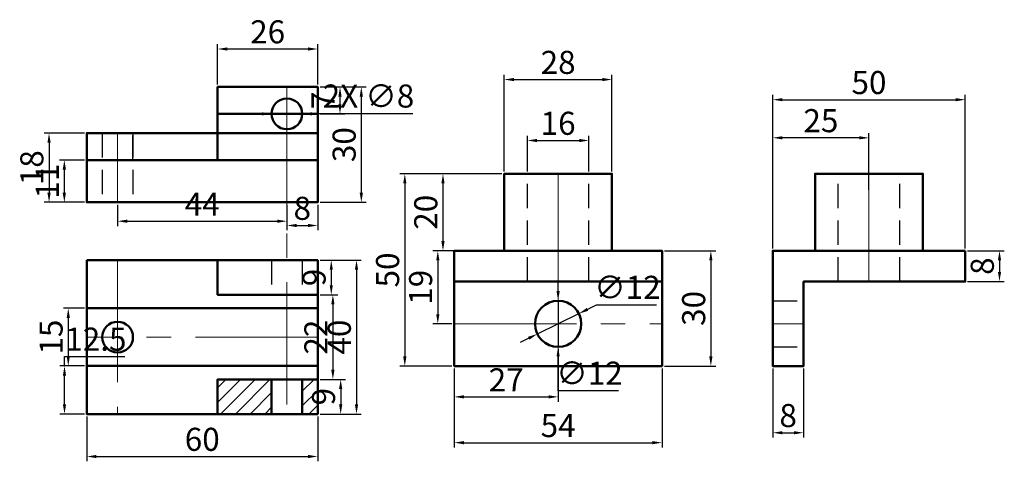
# Model space of a CAD drawing. Units: millimetres. Extents: x 12 to 268, y 574 to 689.
import ezdxf

# ---------------------------------------------------------------- set-up
doc = ezdxf.new("R2010")
doc.units = ezdxf.units.MM
doc.linetypes.add('CENTER', pattern=[50.8, 31.75, -6.35, 6.35, -6.35])
doc.linetypes.add('HIDDEN', pattern=[9.525, 6.35, -3.175])
for name, color, linetype, lineweight in [('M-CNTR', 4, 'CENTER', 18), ('M-DIMS', 2, 'Continuous', 25), ('M-HATC', 8, 'Continuous', 18), ('M-HIDN', 1, 'HIDDEN', 25), ('M-OUTL', 7, 'Continuous', 50)]:
    doc.layers.add(name, color=color, linetype=linetype, lineweight=lineweight)
doc.styles.get("Standard").update_dxf_attribs({"font": 'arial.ttf'})
doc.dimstyles.new('ISO-25', dxfattribs={"dimtxt": 6, "dimasz": 2.5, "dimexe": 1.25, "dimexo": 0.625, "dimtad": 1, "dimtoh": 1, "dimdec": 0, "dimtxsty": 'Standard', "dimcen": 2.5, "dimadec": 0, "dimazin": 0, "dimtfac": 1, "dimtdec": 0, "dimtmove": 0, "dimatfit": 3, "dimfxl": 1, "dimarcsym": 0})

# ---------------------------------------------------------------- blocks, each defined once
blk = doc.blocks.new('*D1')
at = {"layer": 'Defpoints', "color": 0, "transparency": 16777216}
for p in [(89.08, 681.66), (63.08, 671.79), (89.08, 671.79)]:
    blk.add_point(p, dxfattribs=at)
at = {"layer": 'M-DIMS', "color": 0, "lineweight": -2, "transparency": 16777216}
for p, q in [((63.08, 672.42), (63.08, 682.91)), ((65.58, 681.66), (86.58, 681.66)), ((89.08, 672.42), (89.08, 682.91))]:
    blk.add_line(p, q, dxfattribs=at)
at = {"layer": 'M-DIMS', "color": 0, "transparency": 16777216}
for points in [[(65.58, 682.07), (65.58, 681.24), (63.08, 681.66)], [(86.58, 682.07), (86.58, 681.24), (89.08, 681.66)]]:
    blk.add_solid(points, dxfattribs=at)
at = {"layer": 'M-DIMS', "color": 0, "transparency": 16777216, "insert": (76.08, 685.35), "char_height": 6, "attachment_point": 5}
blk.add_mtext('26', dxfattribs=at)
blk = doc.blocks.new('*D2')
at = {"layer": 'Defpoints', "color": 0, "transparency": 16777216}
for p in [(89.08, 671.79), (89.08, 641.79), (100.42, 641.79)]:
    blk.add_point(p, dxfattribs=at)
at = {"layer": 'M-DIMS', "color": 0, "lineweight": -2, "transparency": 16777216}
for p, q in [((89.7, 671.79), (101.67, 671.79)), ((100.42, 669.29), (100.42, 644.29)), ((89.7, 641.79), (101.67, 641.79))]:
    blk.add_line(p, q, dxfattribs=at)
at = {"layer": 'M-DIMS', "color": 0, "transparency": 16777216}
for points in [[(100, 669.29), (100.84, 669.29), (100.42, 671.79)], [(100, 644.29), (100.84, 644.29), (100.42, 641.79)]]:
    blk.add_solid(points, dxfattribs=at)
at = {"layer": 'M-DIMS', "color": 0, "transparency": 16777216, "insert": (96.73, 656.79), "char_height": 6, "attachment_point": 5, "rotation": 90}
blk.add_mtext('30', dxfattribs=at)
blk = doc.blocks.new('*D3')
at = {"layer": 'Defpoints', "color": 0, "transparency": 16777216}
for p in [(29.08, 659.79), (19.26, 641.79), (29.08, 641.79)]:
    blk.add_point(p, dxfattribs=at)
at = {"layer": 'M-DIMS', "color": 0, "lineweight": -2, "transparency": 16777216}
for p, q in [((28.45, 659.79), (18.01, 659.79)), ((19.26, 657.29), (19.26, 644.29)), ((28.45, 641.79), (18.01, 641.79))]:
    blk.add_line(p, q, dxfattribs=at)
at = {"layer": 'M-DIMS', "color": 0, "transparency": 16777216}
for points in [[(18.84, 657.29), (19.68, 657.29), (19.26, 659.79)], [(18.84, 644.29), (19.68, 644.29), (19.26, 641.79)]]:
    blk.add_solid(points, dxfattribs=at)
at = {"layer": 'M-DIMS', "color": 0, "transparency": 16777216, "insert": (15.57, 650.79), "char_height": 6, "attachment_point": 5, "rotation": 90}
blk.add_mtext('18', dxfattribs=at)
blk = doc.blocks.new('*D4')
at = {"layer": 'Defpoints', "color": 0, "transparency": 16777216}
for p in [(29.08, 652.79), (23.23, 641.79), (29.08, 641.79)]:
    blk.add_point(p, dxfattribs=at)
at = {"layer": 'M-DIMS', "color": 0, "lineweight": -2, "transparency": 16777216}
for p, q in [((28.45, 652.79), (21.98, 652.79)), ((23.23, 650.29), (23.23, 644.29)), ((28.45, 641.79), (21.98, 641.79))]:
    blk.add_line(p, q, dxfattribs=at)
at = {"layer": 'M-DIMS', "color": 0, "transparency": 16777216}
for points in [[(22.81, 650.29), (23.65, 650.29), (23.23, 652.79)], [(22.81, 644.29), (23.65, 644.29), (23.23, 641.79)]]:
    blk.add_solid(points, dxfattribs=at)
at = {"layer": 'M-DIMS', "color": 0, "transparency": 16777216, "insert": (19.59, 647.29), "char_height": 6, "attachment_point": 5, "rotation": 90}
blk.add_mtext('11', dxfattribs=at)
blk = doc.blocks.new('*D5')
at = {"layer": 'Defpoints', "color": 0, "transparency": 16777216}
for p in [(37.08, 641.79), (81.08, 641.79), (81.08, 636.88)]:
    blk.add_point(p, dxfattribs=at)
at = {"layer": 'M-DIMS', "color": 0, "lineweight": -2, "transparency": 16777216}
for p, q in [((37.08, 641.17), (37.08, 635.63)), ((81.08, 641.17), (81.08, 635.63)), ((39.58, 636.88), (78.58, 636.88))]:
    blk.add_line(p, q, dxfattribs=at)
at = {"layer": 'M-DIMS', "color": 0, "transparency": 16777216}
for points in [[(39.58, 637.29), (39.58, 636.46), (37.08, 636.88)], [(78.58, 637.29), (78.58, 636.46), (81.08, 636.88)]]:
    blk.add_solid(points, dxfattribs=at)
at = {"layer": 'M-DIMS', "color": 0, "transparency": 16777216, "insert": (59.08, 640.5), "char_height": 6, "attachment_point": 5}
blk.add_mtext('44', dxfattribs=at)
blk = doc.blocks.new('*D6')
at = {"layer": 'Defpoints', "color": 0, "transparency": 16777216}
for p in [(81.08, 641.79), (89.08, 641.79), (89.08, 635.76)]:
    blk.add_point(p, dxfattribs=at)
at = {"layer": 'M-DIMS', "color": 0, "lineweight": -2, "transparency": 16777216}
for p, q in [((81.08, 641.17), (81.08, 634.51)), ((89.08, 641.17), (89.08, 634.51)), ((83.58, 635.76), (86.58, 635.76))]:
    blk.add_line(p, q, dxfattribs=at)
at = {"layer": 'M-DIMS', "color": 0, "transparency": 16777216}
for points in [[(83.58, 636.18), (83.58, 635.35), (81.08, 635.76)], [(86.58, 636.18), (86.58, 635.35), (89.08, 635.76)]]:
    blk.add_solid(points, dxfattribs=at)
at = {"layer": 'M-DIMS', "color": 0, "transparency": 16777216, "insert": (85.08, 639.45), "char_height": 6, "attachment_point": 5}
blk.add_mtext('8', dxfattribs=at)
blk = doc.blocks.new('*D7')
at = {"layer": 'Defpoints', "color": 0, "transparency": 16777216}
for p in [(89.08, 626.74), (89.08, 617.74), (92.61, 617.74)]:
    blk.add_point(p, dxfattribs=at)
at = {"layer": 'M-DIMS', "color": 0, "lineweight": -2, "transparency": 16777216}
for p, q in [((89.7, 626.74), (93.86, 626.74)), ((92.61, 624.24), (92.61, 620.24)), ((89.7, 617.74), (93.86, 617.74))]:
    blk.add_line(p, q, dxfattribs=at)
at = {"layer": 'M-DIMS', "color": 0, "transparency": 16777216}
for points in [[(92.2, 624.24), (93.03, 624.24), (92.61, 626.74)], [(92.2, 620.24), (93.03, 620.24), (92.61, 617.74)]]:
    blk.add_solid(points, dxfattribs=at)
at = {"layer": 'M-DIMS', "color": 0, "transparency": 16777216, "insert": (88.92, 622.24), "char_height": 6, "attachment_point": 5, "rotation": 90}
blk.add_mtext('9', dxfattribs=at)
blk = doc.blocks.new('*D8')
at = {"layer": 'Defpoints', "color": 0, "transparency": 16777216}
for p in [(89.08, 626.74), (89.08, 586.74), (99.17, 586.74)]:
    blk.add_point(p, dxfattribs=at)
at = {"layer": 'M-DIMS', "color": 0, "lineweight": -2, "transparency": 16777216}
for p, q in [((89.7, 626.74), (100.42, 626.74)), ((99.17, 624.24), (99.17, 589.24)), ((89.7, 586.74), (100.42, 586.74))]:
    blk.add_line(p, q, dxfattribs=at)
at = {"layer": 'M-DIMS', "color": 0, "transparency": 16777216}
for points in [[(98.75, 624.24), (99.59, 624.24), (99.17, 626.74)], [(98.75, 589.24), (99.59, 589.24), (99.17, 586.74)]]:
    blk.add_solid(points, dxfattribs=at)
at = {"layer": 'M-DIMS', "color": 0, "transparency": 16777216, "insert": (95.48, 606.74), "char_height": 6, "attachment_point": 5, "rotation": 90}
blk.add_mtext('40', dxfattribs=at)
blk = doc.blocks.new('*D9')
at = {"layer": 'Defpoints', "color": 0, "transparency": 16777216}
for p in [(89.08, 617.74), (89.08, 595.74), (93.03, 595.74)]:
    blk.add_point(p, dxfattribs=at)
at = {"layer": 'M-DIMS', "color": 0, "lineweight": -2, "transparency": 16777216}
for p, q in [((89.7, 617.74), (94.28, 617.74)), ((93.03, 615.24), (93.03, 598.24)), ((89.7, 595.74), (94.28, 595.74))]:
    blk.add_line(p, q, dxfattribs=at)
at = {"layer": 'M-DIMS', "color": 0, "transparency": 16777216}
for points in [[(92.61, 615.24), (93.45, 615.24), (93.03, 617.74)], [(92.61, 598.24), (93.45, 598.24), (93.03, 595.74)]]:
    blk.add_solid(points, dxfattribs=at)
at = {"layer": 'M-DIMS', "color": 0, "transparency": 16777216, "insert": (89.39, 606.74), "char_height": 6, "attachment_point": 5, "rotation": 90}
blk.add_mtext('22', dxfattribs=at)
blk = doc.blocks.new('*D10')
at = {"layer": 'Defpoints', "color": 0, "transparency": 16777216}
for p in [(89.08, 595.74), (89.08, 586.74), (95.06, 586.74)]:
    blk.add_point(p, dxfattribs=at)
at = {"layer": 'M-DIMS', "color": 0, "lineweight": -2, "transparency": 16777216}
for p, q in [((89.7, 595.74), (96.31, 595.74)), ((95.06, 593.24), (95.06, 589.24)), ((89.7, 586.74), (96.31, 586.74))]:
    blk.add_line(p, q, dxfattribs=at)
at = {"layer": 'M-DIMS', "color": 0, "transparency": 16777216}
for points in [[(94.64, 593.24), (95.48, 593.24), (95.06, 595.74)], [(94.64, 589.24), (95.48, 589.24), (95.06, 586.74)]]:
    blk.add_solid(points, dxfattribs=at)
at = {"layer": 'M-DIMS', "color": 0, "transparency": 16777216, "insert": (91.37, 591.24), "char_height": 6, "attachment_point": 5, "rotation": 90}
blk.add_mtext('9', dxfattribs=at)
blk = doc.blocks.new('*D11')
at = {"layer": 'Defpoints', "color": 0, "transparency": 16777216}
for p in [(29.08, 614.24), (24.26, 599.24), (29.08, 599.24)]:
    blk.add_point(p, dxfattribs=at)
at = {"layer": 'M-DIMS', "color": 0, "lineweight": -2, "transparency": 16777216}
for p, q in [((28.45, 614.24), (23.01, 614.24)), ((24.26, 611.74), (24.26, 601.74)), ((28.45, 599.24), (23.01, 599.24))]:
    blk.add_line(p, q, dxfattribs=at)
at = {"layer": 'M-DIMS', "color": 0, "transparency": 16777216}
for points in [[(23.84, 611.74), (24.67, 611.74), (24.26, 614.24)], [(23.84, 601.74), (24.67, 601.74), (24.26, 599.24)]]:
    blk.add_solid(points, dxfattribs=at)
at = {"layer": 'M-DIMS', "color": 0, "transparency": 16777216, "insert": (20.57, 606.74), "char_height": 6, "attachment_point": 5, "rotation": 90}
blk.add_mtext('15', dxfattribs=at)
blk = doc.blocks.new('*D12')
at = {"layer": 'Defpoints', "color": 0, "transparency": 16777216}
for p in [(29.08, 586.74), (89.08, 586.74), (89.08, 575.69)]:
    blk.add_point(p, dxfattribs=at)
at = {"layer": 'M-DIMS', "color": 0, "lineweight": -2, "transparency": 16777216}
for p, q in [((29.08, 586.11), (29.08, 574.44)), ((89.08, 586.11), (89.08, 574.44)), ((31.58, 575.69), (86.58, 575.69))]:
    blk.add_line(p, q, dxfattribs=at)
at = {"layer": 'M-DIMS', "color": 0, "transparency": 16777216}
for points in [[(31.58, 576.11), (31.58, 575.27), (29.08, 575.69)], [(86.58, 576.11), (86.58, 575.27), (89.08, 575.69)]]:
    blk.add_solid(points, dxfattribs=at)
at = {"layer": 'M-DIMS', "color": 0, "transparency": 16777216, "insert": (59.08, 579.38), "char_height": 6, "attachment_point": 5}
blk.add_mtext('60', dxfattribs=at)
blk = doc.blocks.new('*D13')
at = {"layer": 'Defpoints', "color": 0, "transparency": 16777216}
for p in [(124.57, 599.2), (178.57, 599.2), (178.57, 579.29)]:
    blk.add_point(p, dxfattribs=at)
at = {"layer": 'M-DIMS', "color": 0, "lineweight": -2, "transparency": 16777216}
for p, q in [((124.57, 598.57), (124.57, 578.04)), ((178.57, 598.57), (178.57, 578.04)), ((127.07, 579.29), (176.07, 579.29))]:
    blk.add_line(p, q, dxfattribs=at)
at = {"layer": 'M-DIMS', "color": 0, "transparency": 16777216}
for points in [[(127.07, 579.7), (127.07, 578.87), (124.57, 579.29)], [(176.07, 579.7), (176.07, 578.87), (178.57, 579.29)]]:
    blk.add_solid(points, dxfattribs=at)
at = {"layer": 'M-DIMS', "color": 0, "transparency": 16777216, "insert": (151.57, 582.96), "char_height": 6, "attachment_point": 5}
blk.add_mtext('54', dxfattribs=at)
blk = doc.blocks.new('*D14')
at = {"layer": 'Defpoints', "color": 0, "transparency": 16777216}
for p in [(165.57, 673.72), (137.57, 649.2), (165.57, 649.2)]:
    blk.add_point(p, dxfattribs=at)
at = {"layer": 'M-DIMS', "color": 0, "lineweight": -2, "transparency": 16777216}
for p, q in [((137.57, 649.82), (137.57, 674.97)), ((140.07, 673.72), (163.07, 673.72)), ((165.57, 649.82), (165.57, 674.97))]:
    blk.add_line(p, q, dxfattribs=at)
at = {"layer": 'M-DIMS', "color": 0, "transparency": 16777216}
for points in [[(140.07, 674.13), (140.07, 673.3), (137.57, 673.72)], [(163.07, 674.13), (163.07, 673.3), (165.57, 673.72)]]:
    blk.add_solid(points, dxfattribs=at)
at = {"layer": 'M-DIMS', "color": 0, "transparency": 16777216, "insert": (151.57, 677.4), "char_height": 6, "attachment_point": 5}
blk.add_mtext('28', dxfattribs=at)
blk = doc.blocks.new('*D15')
at = {"layer": 'Defpoints', "color": 0, "transparency": 16777216}
for p in [(159.57, 657.87), (143.57, 649.2), (159.57, 649.2)]:
    blk.add_point(p, dxfattribs=at)
at = {"layer": 'M-DIMS', "color": 0, "lineweight": -2, "transparency": 16777216}
for p, q in [((143.57, 649.82), (143.57, 659.12)), ((146.07, 657.87), (157.07, 657.87)), ((159.57, 649.82), (159.57, 659.12))]:
    blk.add_line(p, q, dxfattribs=at)
at = {"layer": 'M-DIMS', "color": 0, "transparency": 16777216}
for points in [[(146.07, 658.28), (146.07, 657.45), (143.57, 657.87)], [(157.07, 658.28), (157.07, 657.45), (159.57, 657.87)]]:
    blk.add_solid(points, dxfattribs=at)
at = {"layer": 'M-DIMS', "color": 0, "transparency": 16777216, "insert": (151.57, 661.56), "char_height": 6, "attachment_point": 5}
blk.add_mtext('16', dxfattribs=at)
blk = doc.blocks.new('*D16')
at = {"layer": 'Defpoints', "color": 0, "transparency": 16777216}
for p in [(137.57, 649.2), (111.72, 599.2), (124.57, 599.2)]:
    blk.add_point(p, dxfattribs=at)
at = {"layer": 'M-DIMS', "color": 0, "lineweight": -2, "transparency": 16777216}
for p, q in [((136.94, 649.2), (110.47, 649.2)), ((111.72, 646.7), (111.72, 601.7)), ((123.94, 599.2), (110.47, 599.2))]:
    blk.add_line(p, q, dxfattribs=at)
at = {"layer": 'M-DIMS', "color": 0, "transparency": 16777216}
for points in [[(111.3, 646.7), (112.14, 646.7), (111.72, 649.2)], [(111.3, 601.7), (112.14, 601.7), (111.72, 599.2)]]:
    blk.add_solid(points, dxfattribs=at)
at = {"layer": 'M-DIMS', "color": 0, "transparency": 16777216, "insert": (108.03, 624.2), "char_height": 6, "attachment_point": 5, "rotation": 90}
blk.add_mtext('50', dxfattribs=at)
blk = doc.blocks.new('*D17')
at = {"layer": 'Defpoints', "color": 0, "transparency": 16777216}
for p in [(137.57, 649.2), (121.64, 629.2), (137.57, 629.2)]:
    blk.add_point(p, dxfattribs=at)
at = {"layer": 'M-DIMS', "color": 0, "lineweight": -2, "transparency": 16777216}
for p, q in [((136.94, 649.2), (120.39, 649.2)), ((121.64, 646.7), (121.64, 631.7)), ((136.94, 629.2), (120.39, 629.2))]:
    blk.add_line(p, q, dxfattribs=at)
at = {"layer": 'M-DIMS', "color": 0, "transparency": 16777216}
for points in [[(121.23, 646.7), (122.06, 646.7), (121.64, 649.2)], [(121.23, 631.7), (122.06, 631.7), (121.64, 629.2)]]:
    blk.add_solid(points, dxfattribs=at)
at = {"layer": 'M-DIMS', "color": 0, "transparency": 16777216, "insert": (117.95, 639.2), "char_height": 6, "attachment_point": 5, "rotation": 90}
blk.add_mtext('20', dxfattribs=at)
blk = doc.blocks.new('*D18')
at = {"layer": 'Defpoints', "color": 0, "transparency": 16777216}
for p in [(124.57, 629.2), (120.3, 610.2), (124.57, 610.2)]:
    blk.add_point(p, dxfattribs=at)
at = {"layer": 'M-DIMS', "color": 0, "lineweight": -2, "transparency": 16777216}
for p, q in [((123.94, 629.2), (119.05, 629.2)), ((120.3, 626.7), (120.3, 612.7)), ((123.94, 610.2), (119.05, 610.2))]:
    blk.add_line(p, q, dxfattribs=at)
at = {"layer": 'M-DIMS', "color": 0, "transparency": 16777216}
for points in [[(119.88, 626.7), (120.72, 626.7), (120.3, 629.2)], [(119.88, 612.7), (120.72, 612.7), (120.3, 610.2)]]:
    blk.add_solid(points, dxfattribs=at)
at = {"layer": 'M-DIMS', "color": 0, "transparency": 16777216, "insert": (116.61, 619.7), "char_height": 6, "attachment_point": 5, "rotation": 90}
blk.add_mtext('19', dxfattribs=at)
blk = doc.blocks.new('*D19')
at = {"layer": 'Defpoints', "color": 0, "transparency": 16777216}
for p in [(156.95, 612.85), (146.18, 607.55)]:
    blk.add_point(p, dxfattribs=at)
at = {"layer": 'M-DIMS', "color": 0, "lineweight": -2, "transparency": 16777216}
for p, q in [((161.44, 615.05), (159.2, 613.95)), ((177.13, 615.05), (161.44, 615.05)), ((146.18, 607.55), (156.95, 612.85)), ((143.94, 606.45), (141.7, 605.35))]:
    blk.add_line(p, q, dxfattribs=at)
at = {"layer": 'M-DIMS', "color": 0, "transparency": 16777216}
for points in [[(159.01, 614.32), (159.38, 613.58), (156.95, 612.85)], [(143.76, 606.82), (144.12, 606.08), (146.18, 607.55)]]:
    blk.add_solid(points, dxfattribs=at)
at = {"layer": 'M-DIMS', "color": 0, "transparency": 16777216, "insert": (169.59, 618.91), "char_height": 6, "attachment_point": 5}
blk.add_mtext('∅12', dxfattribs=at)
blk = doc.blocks.new('*D20')
at = {"layer": 'Defpoints', "color": 0, "transparency": 16777216}
for p in [(178.57, 629.2), (178.57, 599.2), (191.27, 599.2)]:
    blk.add_point(p, dxfattribs=at)
at = {"layer": 'M-DIMS', "color": 0, "lineweight": -2, "transparency": 16777216}
for p, q in [((179.19, 629.2), (192.52, 629.2)), ((191.27, 626.7), (191.27, 601.7)), ((179.19, 599.2), (192.52, 599.2))]:
    blk.add_line(p, q, dxfattribs=at)
at = {"layer": 'M-DIMS', "color": 0, "transparency": 16777216}
for points in [[(190.85, 626.7), (191.68, 626.7), (191.27, 629.2)], [(190.85, 601.7), (191.68, 601.7), (191.27, 599.2)]]:
    blk.add_solid(points, dxfattribs=at)
at = {"layer": 'M-DIMS', "color": 0, "transparency": 16777216, "insert": (187.57, 614.2), "char_height": 6, "attachment_point": 5, "rotation": 90}
blk.add_mtext('30', dxfattribs=at)
blk = doc.blocks.new('*D21')
at = {"layer": 'Defpoints', "color": 0, "transparency": 16777216}
for p in [(257.36, 668.48), (207.36, 629.2), (257.36, 629.2)]:
    blk.add_point(p, dxfattribs=at)
at = {"layer": 'M-DIMS', "color": 0, "lineweight": -2, "transparency": 16777216}
for p, q in [((207.36, 629.82), (207.36, 669.73)), ((209.86, 668.48), (254.86, 668.48)), ((257.36, 629.82), (257.36, 669.73))]:
    blk.add_line(p, q, dxfattribs=at)
at = {"layer": 'M-DIMS', "color": 0, "transparency": 16777216}
for points in [[(209.86, 668.89), (209.86, 668.06), (207.36, 668.48)], [(254.86, 668.89), (254.86, 668.06), (257.36, 668.48)]]:
    blk.add_solid(points, dxfattribs=at)
at = {"layer": 'M-DIMS', "color": 0, "transparency": 16777216, "insert": (232.36, 672.16), "char_height": 6, "attachment_point": 5}
blk.add_mtext('50', dxfattribs=at)
blk = doc.blocks.new('*D22')
at = {"layer": 'Defpoints', "color": 0, "transparency": 16777216}
for p in [(257.36, 629.2), (257.36, 621.2), (266.28, 621.2)]:
    blk.add_point(p, dxfattribs=at)
at = {"layer": 'M-DIMS', "color": 0, "lineweight": -2, "transparency": 16777216}
for p, q in [((257.98, 629.2), (267.53, 629.2)), ((266.28, 626.7), (266.28, 623.7)), ((257.98, 621.2), (267.53, 621.2))]:
    blk.add_line(p, q, dxfattribs=at)
at = {"layer": 'M-DIMS', "color": 0, "transparency": 16777216}
for points in [[(265.87, 626.7), (266.7, 626.7), (266.28, 629.2)], [(265.87, 623.7), (266.7, 623.7), (266.28, 621.2)]]:
    blk.add_solid(points, dxfattribs=at)
at = {"layer": 'M-DIMS', "color": 0, "transparency": 16777216, "insert": (262.59, 625.2), "char_height": 6, "attachment_point": 5, "rotation": 90}
blk.add_mtext('8', dxfattribs=at)
blk = doc.blocks.new('*D23')
at = {"layer": 'Defpoints', "color": 0, "transparency": 16777216}
for p in [(207.36, 658.56), (207.36, 644.43), (232.36, 644.43)]:
    blk.add_point(p, dxfattribs=at)
at = {"layer": 'M-DIMS', "color": 0, "lineweight": -2, "transparency": 16777216}
for p, q in [((207.36, 645.05), (207.36, 659.81)), ((229.86, 658.56), (209.86, 658.56)), ((232.36, 645.05), (232.36, 659.81))]:
    blk.add_line(p, q, dxfattribs=at)
at = {"layer": 'M-DIMS', "color": 0, "transparency": 16777216}
for points in [[(209.86, 658.98), (209.86, 658.15), (207.36, 658.56)], [(229.86, 658.98), (229.86, 658.15), (232.36, 658.56)]]:
    blk.add_solid(points, dxfattribs=at)
at = {"layer": 'M-DIMS', "color": 0, "transparency": 16777216, "insert": (219.86, 662.25), "char_height": 6, "attachment_point": 5}
blk.add_mtext('25', dxfattribs=at)
blk = doc.blocks.new('*D24')
at = {"layer": 'Defpoints', "color": 0, "transparency": 16777216}
for p in [(207.36, 599.2), (215.36, 599.2), (215.36, 581.87)]:
    blk.add_point(p, dxfattribs=at)
at = {"layer": 'M-DIMS', "color": 0, "lineweight": -2, "transparency": 16777216}
for p, q in [((207.36, 598.57), (207.36, 580.62)), ((215.36, 598.57), (215.36, 580.62)), ((209.86, 581.87), (212.86, 581.87))]:
    blk.add_line(p, q, dxfattribs=at)
at = {"layer": 'M-DIMS', "color": 0, "transparency": 16777216}
for points in [[(209.86, 582.29), (209.86, 581.45), (207.36, 581.87)], [(212.86, 582.29), (212.86, 581.45), (215.36, 581.87)]]:
    blk.add_solid(points, dxfattribs=at)
at = {"layer": 'M-DIMS', "color": 0, "transparency": 16777216, "insert": (211.36, 585.56), "char_height": 6, "attachment_point": 5}
blk.add_mtext('8', dxfattribs=at)
blk = doc.blocks.new('*D25')
at = {"layer": 'Defpoints', "color": 0, "transparency": 16777216}
for p in [(89.08, 671.79), (89.08, 664.79), (94.88, 664.79)]:
    blk.add_point(p, dxfattribs=at)
at = {"layer": 'M-DIMS', "color": 0, "lineweight": -2, "transparency": 16777216}
for p, q in [((89.7, 671.79), (96.13, 671.79)), ((94.88, 669.29), (94.88, 667.29)), ((89.7, 664.79), (96.13, 664.79))]:
    blk.add_line(p, q, dxfattribs=at)
at = {"layer": 'M-DIMS', "color": 0, "transparency": 16777216}
for points in [[(94.46, 669.29), (95.29, 669.29), (94.88, 671.79)], [(94.46, 667.29), (95.29, 667.29), (94.88, 664.79)]]:
    blk.add_solid(points, dxfattribs=at)
at = {"layer": 'M-DIMS', "color": 0, "transparency": 16777216, "insert": (91.25, 668.29), "char_height": 6, "attachment_point": 5, "rotation": 90}
blk.add_mtext('7', dxfattribs=at)
blk = doc.blocks.new('*D26')
at = {"layer": 'Defpoints', "color": 0, "transparency": 16777216}
for p in [(23.28, 599.24), (29.08, 599.24), (29.08, 586.74)]:
    blk.add_point(p, dxfattribs=at)
at = {"layer": 'M-DIMS', "color": 0, "lineweight": -2, "transparency": 16777216}
for p, q in [((23.28, 599.24), (23.28, 601.74)), ((23.28, 601.74), (38.97, 601.74)), ((28.45, 599.24), (22.03, 599.24)), ((23.28, 589.24), (23.28, 596.74)), ((28.45, 586.74), (22.03, 586.74))]:
    blk.add_line(p, q, dxfattribs=at)
at = {"layer": 'M-DIMS', "color": 0, "transparency": 16777216}
for points in [[(22.86, 596.74), (23.69, 596.74), (23.28, 599.24)], [(22.86, 589.24), (23.69, 589.24), (23.28, 586.74)]]:
    blk.add_solid(points, dxfattribs=at)
at = {"layer": 'M-DIMS', "color": 0, "transparency": 16777216, "insert": (31.44, 605.43), "char_height": 6, "attachment_point": 5}
blk.add_mtext('12.5', dxfattribs=at)
blk = doc.blocks.new('*D27')
at = {"layer": 'Defpoints', "color": 0, "transparency": 16777216}
for p in [(151.57, 604.2), (124.57, 599.2), (151.57, 591.2)]:
    blk.add_point(p, dxfattribs=at)
at = {"layer": 'M-DIMS', "color": 0, "lineweight": -2, "transparency": 16777216}
for p, q in [((151.57, 603.57), (151.57, 589.95)), ((124.57, 598.57), (124.57, 589.95)), ((127.07, 591.2), (149.07, 591.2))]:
    blk.add_line(p, q, dxfattribs=at)
at = {"layer": 'M-DIMS', "color": 0, "transparency": 16777216}
for points in [[(127.07, 591.62), (127.07, 590.78), (124.57, 591.2)], [(149.07, 591.62), (149.07, 590.78), (151.57, 591.2)]]:
    blk.add_solid(points, dxfattribs=at)
at = {"layer": 'M-DIMS', "color": 0, "transparency": 16777216, "insert": (138.07, 594.84), "char_height": 6, "attachment_point": 5}
blk.add_mtext('27', dxfattribs=at)
blk = doc.blocks.new('*D28')
at = {"layer": 'Defpoints', "color": 0, "transparency": 16777216}
for p in [(77.08, 664.79), (85.08, 664.79)]:
    blk.add_point(p, dxfattribs=at)
at = {"layer": 'M-DIMS', "color": 0, "lineweight": -2, "transparency": 16777216}
for p, q in [((74.58, 664.79), (72.08, 664.79)), ((77.08, 664.79), (85.08, 664.79)), ((90.08, 664.79), (87.58, 664.79)), ((113.85, 664.79), (90.08, 664.79))]:
    blk.add_line(p, q, dxfattribs=at)
at = {"layer": 'M-DIMS', "color": 0, "transparency": 16777216}
for points in [[(74.58, 665.21), (74.58, 664.37), (77.08, 664.79)], [(87.58, 665.21), (87.58, 664.38), (85.08, 664.79)]]:
    blk.add_solid(points, dxfattribs=at)
at = {"layer": 'M-DIMS', "color": 0, "transparency": 16777216, "insert": (102.28, 668.65), "char_height": 6, "attachment_point": 5}
blk.add_mtext('2X ∅8', dxfattribs=at)
blk = doc.blocks.new('*D29')
at = {"layer": 'Defpoints', "color": 0, "transparency": 16777216}
for p in [(151.57, 616.2), (151.57, 604.2)]:
    blk.add_point(p, dxfattribs=at)
at = {"layer": 'M-DIMS', "color": 0, "lineweight": -2, "transparency": 16777216}
for p, q in [((151.57, 618.7), (151.57, 621.2)), ((151.57, 616.2), (151.57, 604.2)), ((151.57, 592.74), (151.57, 601.7)), ((167.25, 592.74), (151.57, 592.74))]:
    blk.add_line(p, q, dxfattribs=at)
at = {"layer": 'M-DIMS', "color": 0, "transparency": 16777216}
for points in [[(151.98, 618.7), (151.15, 618.7), (151.57, 616.2)], [(151.98, 601.7), (151.15, 601.7), (151.57, 604.2)]]:
    blk.add_solid(points, dxfattribs=at)
at = {"layer": 'M-DIMS', "color": 0, "transparency": 16777216, "insert": (159.72, 596.59), "char_height": 6, "attachment_point": 5}
blk.add_mtext('∅12', dxfattribs=at)

msp = doc.modelspace()

# ---------------------------------------------------------------- hatches: boundary and pattern name
at = {"layer": 'M-HATC'}
h = msp.add_hatch(dxfattribs=at)
h.set_pattern_fill('ANSI31', color=256, scale=0.85)
h.paths.add_polyline_path([(77.08, 595.74), (63.08, 595.74), (63.08, 586.74), (77.08, 586.74)])
h.paths.add_polyline_path([(89.08, 595.74), (85.08, 595.74), (85.08, 586.74), (89.08, 586.74)])

# ---------------------------------------------------------------- linework, layer by layer
at = {"layer": 'M-CNTR'}
for p, q in [((81.08, 671.79), (81.08, 586.74)), ((37.08, 659.79), (37.08, 641.79)), ((232.36, 621.2), (232.36, 649.2)), ((37.08, 626.74), (37.08, 586.74)), ((124.57, 610.2), (178.57, 610.2)), ((207.36, 610.2), (215.36, 610.2)), ((89.08, 606.74), (29.08, 606.74))]:
    msp.add_line(p, q, dxfattribs=at)
msp.add_lwpolyline([(151.57, 599.2), (151.57, 629.2), (151.57, 649.2)], dxfattribs=at)
at = {"layer": 'M-HIDN'}
for p, q in [((33.08, 659.79), (33.08, 641.79)), ((143.57, 621.2), (143.57, 649.2)), ((159.57, 621.2), (159.57, 649.2)), ((224.36, 621.2), (224.36, 649.2)), ((240.36, 621.2), (240.36, 649.2)), ((77.08, 626.74), (77.08, 617.74)), ((85.08, 626.74), (85.08, 617.74)), ((207.36, 616.2), (215.36, 616.2)), ((207.36, 604.2), (215.36, 604.2))]:
    msp.add_line(p, q, dxfattribs=at)
msp.add_lwpolyline([(41.08, 652.79), (41.08, 659.79), (41.08, 641.79)], dxfattribs=at)
at = {"layer": 'M-OUTL'}
for p, q in [((63.08, 664.79), (89.08, 664.79)), ((29.08, 652.79), (63.08, 652.79)), ((124.57, 621.2), (178.57, 621.2)), ((29.08, 614.24), (89.08, 614.24)), ((89.08, 599.24), (29.08, 599.24)), ((77.08, 595.74), (77.08, 586.74)), ((85.08, 595.74), (85.08, 586.74))]:
    msp.add_line(p, q, dxfattribs=at)
for points in [[(89.08, 652.79), (63.08, 652.79), (63.08, 671.79), (89.08, 671.79), (89.08, 641.79), (29.08, 641.79), (29.08, 659.79), (63.08, 659.79), (89.08, 659.79)], [(137.57, 629.2), (137.57, 649.2), (165.57, 649.2), (165.57, 629.2)], [(218.36, 629.2), (218.36, 649.2), (246.36, 649.2), (246.36, 629.2)], [(63.08, 626.74), (63.08, 617.74), (89.08, 617.74)], [(89.08, 595.74), (63.08, 595.74), (63.08, 586.74)]]:
    msp.add_lwpolyline(points, dxfattribs=at)
for points in [[(124.57, 629.2), (124.57, 599.2), (178.57, 599.2), (178.57, 629.2)], [(257.36, 629.2), (257.36, 621.2), (215.36, 621.2), (215.36, 599.2), (207.36, 599.2), (207.36, 629.2)], [(29.08, 626.74), (89.08, 626.74), (89.08, 586.74), (29.08, 586.74)]]:
    msp.add_lwpolyline(points, close=True, dxfattribs=at)
for centre, radius in [((81.08, 664.79), 4), ((151.57, 610.2), 6), ((37.08, 606.74), 4)]:
    msp.add_circle(centre, radius, dxfattribs=at)

# ---------------------------------------------------------------- dimensions: what is measured, and where the dimension line sits
at = {"layer": 'M-DIMS'}
for base, p1, p2, override, picture, middle in [((89.08, 681.66), (63.08, 671.79), (89.08, 671.79), {"dimclrd": 0, "dimclre": 0, "dimclrt": 0}, '*D1', (76.08, 685.35)), ((165.57, 673.72), (137.57, 649.2), (165.57, 649.2), {"dimclrd": 0, "dimclre": 0, "dimclrt": 0}, '*D14', (151.57, 677.4)), ((257.36, 668.48), (207.36, 629.2), (257.36, 629.2), {"dimclrd": 0, "dimclre": 0, "dimclrt": 0}, '*D21', (232.36, 672.16)), ((159.57, 657.87), (143.57, 649.2), (159.57, 649.2), {"dimclrd": 0, "dimclre": 0, "dimclrt": 0}, '*D15', (151.57, 661.56)), ((207.36, 658.56), (232.36, 644.43), (207.36, 644.43), {"dimclrd": 0, "dimclre": 0, "dimclrt": 0}, '*D23', (219.86, 662.25)), ((81.08, 636.88), (37.08, 641.79), (81.08, 641.79), {"dimclrd": 0, "dimclre": 0, "dimclrt": 0}, '*D5', (59.08, 640.5)), ((89.08, 635.76), (81.08, 641.79), (89.08, 641.79), {"dimclrd": 0, "dimclre": 0, "dimclrt": 0}, '*D6', (85.08, 639.45)), ((151.57, 591.2), (124.57, 599.2), (151.57, 604.2), {"dimdec": 0, "dimlfac": 1, "dimrnd": 0, "dimzin": 0, "dimdsep": 46, "dimlunit": 2}, '*D27', (138.07, 594.84)), ((178.57, 579.29), (124.57, 599.2), (178.57, 599.2), {"dimclrd": 0, "dimclre": 0, "dimclrt": 0}, '*D13', (151.57, 582.96)), ((215.36, 581.87), (207.36, 599.2), (215.36, 599.2), {"dimclrd": 0, "dimclre": 0, "dimclrt": 0}, '*D24', (211.36, 585.56)), ((89.08, 575.69), (29.08, 586.74), (89.08, 586.74), {"dimclrd": 0, "dimclre": 0, "dimclrt": 0}, '*D12', (59.08, 579.38))]:
    dim = msp.add_linear_dim(base=base, p1=p1, p2=p2, dimstyle='ISO-25', override=override, dxfattribs=at)
    dim.commit()
    dim.dimension.update_dxf_attribs({"geometry": picture, "text_midpoint": middle})
dim = msp.add_diameter_dim_2p(p1=(77.08, 664.79), p2=(85.08, 664.79), text='2X <>', dimstyle='ISO-25', override={"dimdec": 0, "dimlfac": 1, "dimrnd": 0, "dimzin": 0, "dimdsep": 46, "dimlunit": 2}, dxfattribs=at)
dim.commit()
dim.dimension.update_dxf_attribs({"geometry": '*D28', "text_midpoint": (90.08, 664.79)})
for base, p1, p2, override, picture, middle in [((94.88, 664.79), (89.08, 671.79), (89.08, 664.79), {"dimdec": 0, "dimlfac": 1, "dimrnd": 0, "dimzin": 0, "dimdsep": 46, "dimlunit": 2}, '*D25', (91.25, 668.29)), ((100.42, 641.79), (89.08, 671.79), (89.08, 641.79), {"dimclrd": 0, "dimclre": 0, "dimclrt": 0}, '*D2', (96.73, 656.79)), ((19.26, 641.79), (29.08, 659.79), (29.08, 641.79), {"dimclrd": 0, "dimclre": 0, "dimclrt": 0}, '*D3', (15.57, 650.79)), ((23.23, 641.79), (29.08, 652.79), (29.08, 641.79), {"dimclrd": 0, "dimclre": 0, "dimclrt": 0}, '*D4', (19.59, 647.29)), ((111.72, 599.2), (137.57, 649.2), (124.57, 599.2), {"dimclrd": 0, "dimclre": 0, "dimclrt": 0}, '*D16', (108.03, 624.2)), ((121.64, 629.2), (137.57, 649.2), (137.57, 629.2), {"dimclrd": 0, "dimclre": 0, "dimclrt": 0}, '*D17', (117.95, 639.2)), ((120.3, 610.2), (124.57, 629.2), (124.57, 610.2), {"dimclrd": 0, "dimclre": 0, "dimclrt": 0}, '*D18', (116.61, 619.7)), ((191.27, 599.2), (178.57, 629.2), (178.57, 599.2), {"dimclrd": 0, "dimclre": 0, "dimclrt": 0}, '*D20', (187.57, 614.2)), ((266.28, 621.2), (257.36, 629.2), (257.36, 621.2), {"dimclrd": 0, "dimclre": 0, "dimclrt": 0}, '*D22', (262.59, 625.2)), ((92.61, 617.74), (89.08, 626.74), (89.08, 617.74), {"dimclrd": 0, "dimclre": 0, "dimclrt": 0}, '*D7', (88.92, 622.24)), ((99.17, 586.74), (89.08, 626.74), (89.08, 586.74), {"dimclrd": 0, "dimclre": 0, "dimclrt": 0}, '*D8', (95.48, 606.74)), ((93.03, 595.74), (89.08, 617.74), (89.08, 595.74), {"dimclrd": 0, "dimclre": 0, "dimclrt": 0}, '*D9', (89.39, 606.74)), ((24.26, 599.24), (29.08, 614.24), (29.08, 599.24), {"dimclrd": 0, "dimclre": 0, "dimclrt": 0}, '*D11', (20.57, 606.74)), ((23.28, 599.24), (29.08, 586.74), (29.08, 599.24), {"dimdec": 1, "dimlfac": 1, "dimrnd": 0, "dimzin": 0, "dimdsep": 46, "dimlunit": 2}, '*D26', (31.44, 605.43)), ((95.06, 586.74), (89.08, 595.74), (89.08, 586.74), {"dimclrd": 0, "dimclre": 0, "dimclrt": 0}, '*D10', (91.37, 591.24))]:
    dim = msp.add_linear_dim(base=base, p1=p1, p2=p2, angle=90, dimstyle='ISO-25', override=override, dxfattribs=at)
    dim.commit()
    dim.dimension.update_dxf_attribs({"geometry": picture, "text_midpoint": middle})
dim = msp.add_diameter_dim_2p(p1=(146.18, 607.55), p2=(156.95, 612.85), dimstyle='ISO-25', override={"dimclrd": 0, "dimclre": 0, "dimclrt": 0}, dxfattribs=at)
dim.commit()
dim.dimension.update_dxf_attribs({"geometry": '*D19', "text_midpoint": (169.59, 618.91)})
dim = msp.add_diameter_dim_2p(p1=(151.57, 616.2), p2=(151.57, 604.2), dimstyle='ISO-25', override={"dimdec": 0, "dimlfac": 1, "dimrnd": 0, "dimzin": 0, "dimdsep": 46, "dimlunit": 2}, dxfattribs=at)
dim.commit()
dim.dimension.update_dxf_attribs({"geometry": '*D29', "text_midpoint": (159.72, 592.74), "dimtype": 163})

doc.saveas('drawing.dxf')
